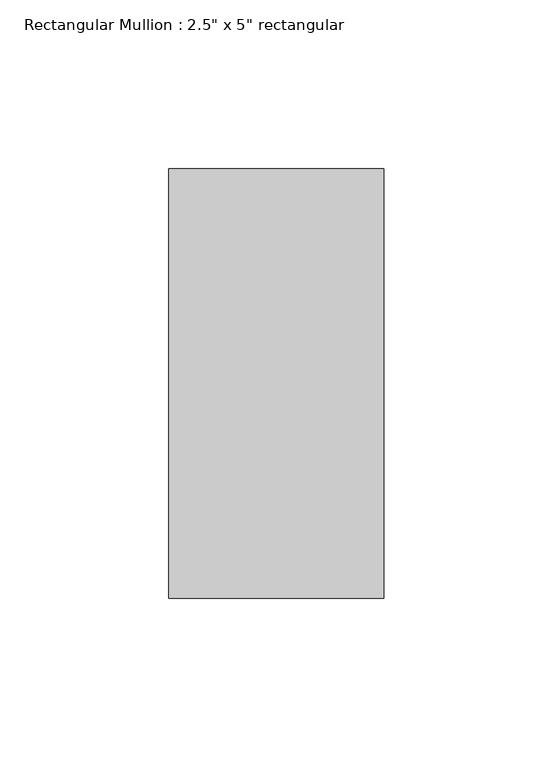
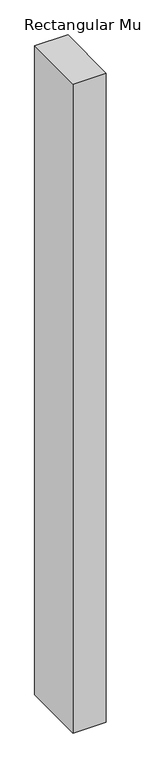
"""IFC4 building model written with IfcOpenShell, lengths in millimetres: member geometry."""

from ifc_helpers import new_model, si_unit, frame, origin, place, context, project, spatial, polyline, outline, extrude, source, transform, mapped, element, save


def member_ae54c2fa(model_context):
    return source(origin(), model_context, "Body", "SweptSolid", [
        extrude(outline(polyline([(31.75, 63.5), (31.75, -63.5), (-31.75, -63.5), (-31.75, 63.5), (31.75, 63.5)])), frame((0.0, 0.0, -1312.0463864), z_axis=(0.0, 0.0, 1.0), x_axis=(1.0, 0.0, 0.0)), (0.0, 0.0, 1.0), 1312.0463864),
    ])


if __name__ == "__main__":
    model = new_model("IFC4")
    model_context = context("Model", 3, world=origin())
    ifc_project = project(units=[si_unit("LENGTHUNIT", "METRE", prefix="MILLI")], contexts=[model_context])
    site = spatial("IfcSite", under=ifc_project)
    building = spatial("IfcBuilding", under=site)
    placement = place(None, origin())
    member_shape = member_ae54c2fa(model_context)
    element("IfcMember", 1, ObjectType="Rectangular Mullion : 2.5\" x 5\" rectangular", at=placement, inside=building, context=model_context, shape_type="MappedRepresentation", body=[
        mapped(member_shape, transform((0.0, 0.0, 0.0), x_axis=(1.0, 0.0, 0.0), y_axis=(0.0, 1.0, 0.0), z_axis=(0.0, 0.0, 1.0))),
    ])
    save(model, "model.ifc")

# Revit data of these elements
# Type "Rectangular Mullion : 2.5\" x 5\" rectangular"
#   built-in parameter 1007304 = 0.416667 (stored number, unit not read)
#   built-in parameter 1007301 = 0.104167 (stored number, unit not read)
#   built-in parameter 1007300 = 0.104167 (stored number, unit not read)
# Element 1 (IfcMember, "Rectangular Mullion : 2.5\" x 5\" rectangular")
#   Materials on its faces: "Aluminum"
# Materials
#   "Aluminum": class "Metal", colour RGB 247 247 247, transparency 0, Description = "Aluminum 6061", Cost = 0
